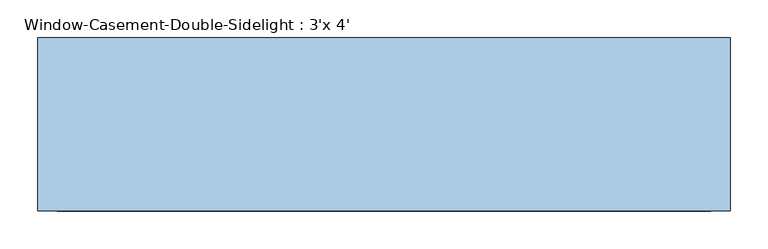
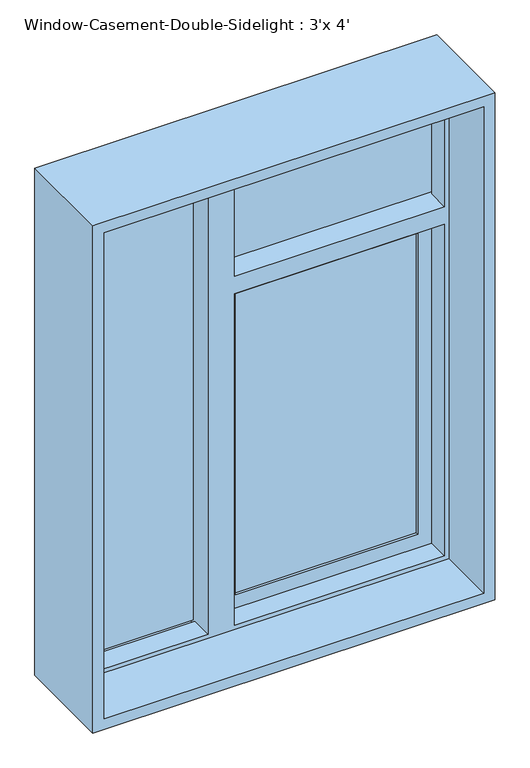
"""IFC4 building model written with IfcOpenShell, lengths in millimetres: window geometry, Window-Casement-Double-Sidelight : 3'x 4'."""

from ifc_helpers import new_model, si_unit, frame, origin, place, context, project, spatial, polyline, outline, extrude, faceted_brep, source, transform, mapped, element, save


def window_casement_double_sidelight_3_x_4_30e8e43c(model_context):
    return source(origin(), model_context, "Body", "SolidModel", [
        extrude(outline(polyline([(389.9296875, 98.425), (-24.1696875, 98.425), (-24.1696875, 111.125), (389.9296875, 111.125), (389.9296875, 98.425)])), frame((0.0, 0.0, 981.6703125), z_axis=(0.0, 0.0, 1.0), x_axis=(1.0, 0.0, 0.0)), (0.0, 0.0, 1.0), 723.3642187),
        extrude(outline(polyline([(389.9296875, 85.725), (389.9296875, 79.375), (-24.1696875, 79.375), (-24.1696875, 85.725), (389.9296875, 85.725)])), frame((0.0, 0.0, 981.6703125), z_axis=(0.0, 0.0, 1.0), x_axis=(1.0, 0.0, 0.0)), (0.0, 0.0, 1.0), 723.3642187),
        extrude(outline(polyline([(-116.84, 98.425), (-116.84, 92.075), (-431.8, 92.075), (-431.8, 98.425), (-116.84, 98.425)])), frame((0.0, 0.0, 949.9203125), z_axis=(0.0, 0.0, 1.0), x_axis=(1.0, 0.0, 0.0)), (0.0, 0.0, 1.0), 1158.2796875),
        extrude(outline(polyline([(-116.84, 85.725), (-116.84, 79.375), (-431.8, 79.375), (-431.8, 85.725), (-116.84, 85.725)])), frame((0.0, 0.0, 949.9203125), z_axis=(0.0, 0.0, 1.0), x_axis=(1.0, 0.0, 0.0)), (0.0, 0.0, 1.0), 1158.2796875),
        extrude(outline(polyline([(431.8, 85.725), (431.8, 79.375), (-66.04, 79.375), (-66.04, 85.725), (431.8, 85.725)])), frame((0.0, 0.0, 1788.7751563), z_axis=(0.0, 0.0, 1.0), x_axis=(1.0, 0.0, 0.0)), (0.0, 0.0, 1.0), 319.4248438),
        extrude(outline(polyline([(431.8, 98.425), (431.8, 92.075), (-66.04, 92.075), (-66.04, 98.425), (431.8, 98.425)])), frame((0.0, 0.0, 1788.7751563), z_axis=(0.0, 0.0, 1.0), x_axis=(1.0, 0.0, 0.0)), (0.0, 0.0, 1.0), 319.4248438),
        faceted_brep([(-431.8, 73.025, 2108.2), (-431.8, 114.3, 2108.2), (431.8, 114.3, 2108.2), (431.8, 73.025, 2108.2), (-66.04, 73.025, 2108.2), (-66.04, 111.125, 2108.2), (-116.84, 111.125, 2108.2), (-116.84, 73.025, 2108.2), (-421.6796875, 22.225, 2098.0796875), (-421.6796875, 73.025, 2098.0796875), (-116.84, 73.025, 2098.0796875), (-116.84, 22.225, 2098.0796875), (421.6796875, 73.025, 2098.0796875), (421.6796875, 22.225, 2098.0796875), (-55.9196875, 22.225, 2098.0796875), (-55.9196875, 73.025, 2098.0796875), (-431.8, -114.3, 2108.2), (-431.8, 22.225, 2108.2), (431.8, 22.225, 2108.2), (431.8, -114.3, 2108.2), (-457.2, 114.3, 2133.6), (-457.2, -114.3, 2133.6), (457.2, -114.3, 2133.6), (457.2, 114.3, 2133.6), (431.8, 114.3, 939.8), (431.8, 73.025, 939.8), (431.8, 73.025, 1746.9048438), (431.8, 111.125, 1746.9048438), (431.8, 111.125, 1788.7751563), (431.8, 73.025, 1788.7751563), (421.6796875, 73.025, 1788.7751563), (421.6796875, 22.225, 1788.7751563), (421.6796875, 73.025, 949.9203125), (421.6796875, 22.225, 949.9203125), (421.6796875, 22.225, 1746.9048438), (421.6796875, 73.025, 1746.9048438), (431.8, 22.225, 939.8), (431.8, -114.3, 939.8), (457.2, -114.3, 914.4), (457.2, 114.3, 914.4), (-431.8, 114.3, 939.8), (-431.8, 73.025, 939.8), (-116.84, 73.025, 939.8), (-116.84, 111.125, 939.8), (-66.04, 111.125, 939.8), (-66.04, 73.025, 939.8), (-55.9196875, 73.025, 949.9203125), (-55.9196875, 22.225, 949.9203125), (-421.6796875, 73.025, 949.9203125), (-421.6796875, 22.225, 949.9203125), (-116.84, 22.225, 949.9203125), (-116.84, 73.025, 949.9203125), (-431.8, 22.225, 939.8), (-431.8, -114.3, 939.8), (-457.2, -114.3, 914.4), (-457.2, 114.3, 914.4), (-55.9196875, 73.025, 1788.7751563), (-66.04, 73.025, 1788.7751563), (-66.04, 73.025, 1746.9048438), (-55.9196875, 73.025, 1746.9048438), (-55.9196875, 22.225, 1788.7751563), (-55.9196875, 22.225, 1746.9048438), (-66.04, 111.125, 1788.7751563), (-66.04, 111.125, 1746.9048438)], [[[0, 1, 2, 3, 4, 5, 6, 7]], [[8, 9, 10, 11]], [[12, 13, 14, 15]], [[16, 17, 18, 19]], [[20, 21, 22, 23]], [[3, 2, 24, 25, 26, 27, 28, 29]], [[13, 12, 30, 31]], [[32, 33, 34, 35]], [[19, 18, 36, 37]], [[23, 22, 38, 39]], [[25, 24, 40, 41, 42, 43, 44, 45]], [[33, 32, 46, 47]], [[48, 49, 50, 51]], [[37, 36, 52, 53]], [[39, 38, 54, 55]], [[1, 0, 41, 40]], [[12, 15, 56, 57, 4, 3, 29, 30]], [[46, 32, 35, 26, 25, 45, 58, 59]], [[41, 0, 7, 10, 9, 48, 51, 42]], [[9, 8, 49, 48]], [[17, 52, 36, 18], [13, 31, 60, 14], [33, 47, 61, 34], [49, 8, 11, 50]], [[17, 16, 53, 52]], [[22, 21, 54, 38], [16, 19, 37, 53]], [[21, 20, 55, 54]], [[20, 23, 39, 55], [2, 1, 40, 24]], [[43, 6, 5, 62, 28, 27, 63, 44]], [[6, 43, 42, 51, 50, 11, 10, 7]], [[15, 14, 60, 56]], [[47, 46, 59, 61]], [[5, 4, 57, 62]], [[45, 44, 63, 58]], [[63, 27, 26, 35, 34, 61, 59, 58]], [[28, 62, 57, 56, 60, 31, 30, 29]]]),
        extrude(outline(polyline([(1746.9048438, 431.8), (1746.9048438, -66.04), (939.8, -66.04), (939.8, 431.8), (1746.9048438, 431.8)]), holes=[polyline([(981.6703125, 389.9296875), (981.6703125, -24.1696875), (1705.0345313, -24.1696875), (1705.0345313, 389.9296875), (981.6703125, 389.9296875)])]), frame((0.0, 73.025, 0.0), z_axis=(0.0, 1.0, 0.0), x_axis=(0.0, 0.0, 1.0)), (0.0, 0.0, 1.0), 31.75),
    ])


if __name__ == "__main__":
    model = new_model("IFC4")
    model_context = context("Model", 3, world=origin())
    ifc_project = project(units=[si_unit("LENGTHUNIT", "METRE", prefix="MILLI")], contexts=[model_context])
    site = spatial("IfcSite", under=ifc_project)
    building = spatial("IfcBuilding", under=site)
    placement = place(None, origin())
    window_casement_double_sidelight_3_x_4_shape = window_casement_double_sidelight_3_x_4_30e8e43c(model_context)
    element("IfcWindow", 1, ObjectType="Window-Casement-Double-Sidelight : 3'x 4'", at=placement, inside=building, context=model_context, shape_type="MappedRepresentation", body=[
        mapped(window_casement_double_sidelight_3_x_4_shape, transform((0.0, 0.0, 0.0), x_axis=(1.0, 0.0, 0.0), y_axis=(0.0, 1.0, 0.0), z_axis=(0.0, 0.0, 1.0))),
    ])
    save(model, "model.ifc")

# Revit data of these elements
# Type "Window-Casement-Double-Sidelight : 3'x 4'"
#   Type Mark = "22"
#   Fire Rating = "0.5h"
#   Assembly Code = "B2020100"
#   Analytic Construction = "Double glazing - domestic"
#   Window Inset [instance default] = 0' - 0 5/8"
#   Wall Thickness [instance default] = 0' - 6"
#   Visual Light Transmittance = 0.81
#   Transom Height Ratio = 0.3
#   Transom Height = 1' - 2.4"
#   Thermal Resistance (R) = 1.8146 (h·ft²·°F)/BTU
#   Solar Heat Gain Coefficient = 0.76
#   Side Width = 1' - 2.4"
#   Rough Width = 3' - 0 1/2"
#   Rough Height = 4' - 0 1/2"
#   Opening Window Width = 1' - 9.6"
#   Opening Window Height = 2' - 9.6"
#   Heat Transfer Coefficient (U) = 0.5511 BTU/(h·ft²·°F)
#   Height = 4' - 0"
#   Frame Gap 3 [instance default] = 0' - 1 83/128"
#   Frame Gap 2 [instance default] = 0' - 0 5/8"
#   Frame Gap 1 = 0' - 1 51/128"
#   Default Sill Height = 3' - 0"
#   Width = 3' - 0"
#   Frame Material = Metal - Aluminum
#   Glass Panel Material = Glass
#   Wall Closure = (empty or 0)
# Element 1 (IfcWindow, "Window-Casement-Double-Sidelight : 3'x 4'")
#   Wall Thickness = 0' - 9"
#   Materials on its faces: "Metal - Aluminum", "Glass"
# Materials
#   "Metal - Aluminum": class "Metal", colour RGB 247 247 247, transparency 0
#   "Glass": class "Glass", colour RGB 0 128 192, transparency 0.75, Description = "Soda Lime Glass", Cost = 0
